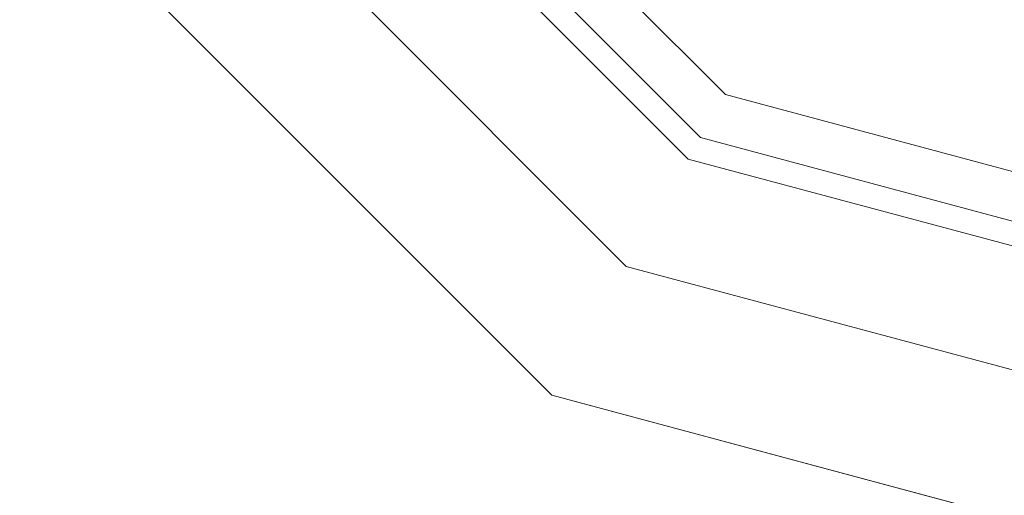
# Model space of a CAD drawing. Units: inches. Extents: x 375 to 1122, y 27 to 1069.
# Tile 133 of 155: x 720.668 to 725.559, y 903.908 to 906.27. Entities that reach past the tile are written whole.
import ezdxf

# ---------------------------------------------------------------- set-up
doc = ezdxf.new("R2010")
doc.units = ezdxf.units.IN
doc.layers.add('A-ANNO-DIMS', color=2, linetype='Continuous', lineweight=18)
doc.layers.add('Furniture', color=30, linetype='Continuous', lineweight=18)
doc.styles.get("Standard").update_dxf_attribs({"font": 'arial.ttf'})
doc.dimstyles.new('ISO-25', dxfattribs={"dimtxt": 12, "dimasz": 2.5, "dimexe": 1.5, "dimexo": 1.5, "dimtad": 1, "dimdec": 1, "dimlunit": 3, "dimtxsty": 'Standard', "dimblk": 'ARCHTICK', "dimcen": 2.5, "dimadec": 0, "dimazin": 0, "dimtfac": 1, "dimtdec": 1, "dimtmove": 0, "dimatfit": 3, "dimfxl": 1.5, "dimfxlon": 1, "dimarcsym": 0})

# ---------------------------------------------------------------- blocks, each defined once
blk = doc.blocks.new('A$C403C54AD')
at = {"linetype": 'ByBlock', "invisible_edges": 5}
for points in [[(0.81594, 0.97759, -0.02585), (0.72796, 1.02838, -0.02585), (0.72796, 1.02838, -0.02585), (0.82955, 1.02838, -0.02585)], [(0.77876, 0.94041, -0.02585), (0.72796, 1.02838, -0.02585), (0.72796, 1.02838, -0.02585), (0.81594, 0.97759, -0.02585)], [(0.81061, 0.98067, -0.04278), (0.81861, 0.97605, -0.03355), (0.83263, 1.02838, -0.03355), (0.82339, 1.02838, -0.04278)], [(0.83194, 0.96835, -0.0197), (0.81594, 0.97759, -0.02585), (0.82955, 1.02838, -0.02585), (0.84802, 1.02838, -0.0197)], [(0.81861, 0.97605, -0.03355), (0.84793, 0.95912, -0.02431), (0.86649, 1.02838, -0.02431), (0.83263, 1.02838, -0.03355)], [(0.84793, 0.95912, -0.0197), (0.83194, 0.96835, -0.0197), (0.84802, 1.02838, -0.0197), (0.86649, 1.02838, -0.0197)], [(0.77568, 0.94574, -0.04278), (0.7803, 0.93774, -0.03355), (0.81861, 0.97605, -0.03355), (0.81061, 0.98067, -0.04278)], [(0.78799, 0.92441, -0.0197), (0.77876, 0.94041, -0.02585), (0.81594, 0.97759, -0.02585), (0.83194, 0.96835, -0.0197)], [(0.7803, 0.93774, -0.03355), (0.79723, 0.90841, -0.02431), (0.84793, 0.95912, -0.02431), (0.81861, 0.97605, -0.03355)], [(0.79723, 0.90841, -0.0197), (0.78799, 0.92441, -0.0197), (0.83194, 0.96835, -0.0197), (0.84793, 0.95912, -0.0197)]]:
    blk.add_3dface(points, dxfattribs=at)
at = {"linetype": 'ByBlock'}
for points in [[(0.84793, 0.95912, -0.02431), (0.84793, 0.95912, -0.0197), (0.86649, 1.02838, -0.0197), (0.86649, 1.02838, -0.02431)], [(0.79723, 0.90841, -0.02431), (0.79723, 0.90841, -0.0197), (0.84793, 0.95912, -0.0197), (0.84793, 0.95912, -0.02431)]]:
    blk.add_3dface(points, dxfattribs=at)
blk = doc.blocks.new('_ArchTick')
at = {"color": 0, "linetype": 'ByBlock', "const_width": 0.15}
blk.add_lwpolyline([(-0.5, -0.5), (0.5, 0.5)], dxfattribs=at)
blk = doc.blocks.new('*D73')
at = {"layer": 'A-ANNO-DIMS', "color": 0, "lineweight": -2, "transparency": 16777216}
for p, q in [((686.7573, 932.4277), (686.7573, 929.4277)), ((770.7573, 932.4277), (770.7573, 929.4277)), ((686.7573, 930.9277), (770.7573, 930.9277)), ((770.7573, 930.9277), (987.6096, 930.9277))]:
    blk.add_line(p, q, dxfattribs=at)
at = {"layer": 'Defpoints', "color": 0, "transparency": 16777216}
for p in [(686.7573, 943.5277), (770.7573, 943.5277), (770.7573, 930.9277)]:
    blk.add_point(p, dxfattribs=at)
at = {"layer": 'A-ANNO-DIMS', "color": 0, "lineweight": -2, "transparency": 16777216, "xscale": 2.5, "yscale": 2.5, "zscale": 2.5, "rotation": 180}
blk.add_blockref('_ArchTick', (686.7573, 930.9277), dxfattribs=at)
at = {"layer": 'A-ANNO-DIMS', "color": 0, "lineweight": -2, "transparency": 16777216, "xscale": 2.5, "yscale": 2.5, "zscale": 2.5}
blk.add_blockref('_ArchTick', (770.7573, 930.9277), dxfattribs=at)
at = {"layer": 'A-ANNO-DIMS', "color": 0, "transparency": 16777216, "insert": (880.4335, 937.7573), "char_height": 12, "attachment_point": 5}
blk.add_mtext('2-PANEL SLIDER 7\'-0" TYP.', dxfattribs=at)

msp = doc.modelspace()

# ---------------------------------------------------------------- block references
at = {"layer": 'Furniture', "xscale": 39.9918517141215, "yscale": 39.9918517141215, "zscale": 39.9918517141215, "rotation": 270}
msp.add_blockref('A$C403C54AD', (684.9549, 938.3156, 0.024), dxfattribs=at)

# ---------------------------------------------------------------- dimensions: what is measured, and where the dimension line sits
at = {"layer": 'A-ANNO-DIMS'}
dim = msp.add_linear_dim(base=(770.7573, 930.9277), p1=(686.7573, 943.5277), p2=(770.7573, 943.5277), text='2-PANEL SLIDER <> TYP.', dimstyle='ISO-25', override={"dimdec": 1, "dimlfac": 1, "dimrnd": 0, "dimzin": 1, "dimdsep": 46, "dimlunit": 4, "dimfrac": 2}, dxfattribs=at)
dim.commit()
dim.dimension.update_dxf_attribs({"geometry": '*D73', "text_midpoint": (880.4335, 937.7573)})

doc.saveas('drawing.dxf')
